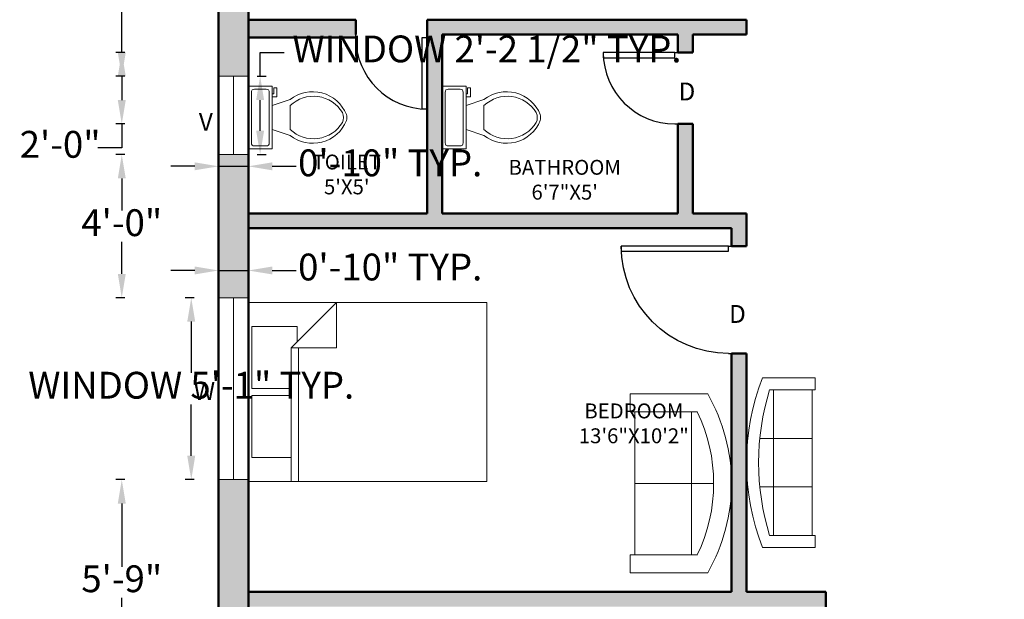
# Model space of a CAD drawing. Units: inches. Extents: x 2568 to 3190, y 746 to 1467.
# Tile 5 of 7: x 2568 to 2898, y 1073 to 1267. Entities that reach past the tile are written whole.
import ezdxf

# ---------------------------------------------------------------- set-up
doc = ezdxf.new("R2010")
doc.units = ezdxf.units.IN
for name, color, linetype, lineweight in [('A-ANNO-DIMS', 2, 'Continuous', 18), ('A-ANNO-TEXT', 7, 'Continuous', 18), ('A-AREA-IDEN', 7, 'Continuous', 25), ('A-DOOR', 3, 'Continuous', 25), ('A-FLOR-FIXT', 9, 'Continuous', 20), ('A-FURN', 8, 'Continuous', 18), ('A-GLAZ', 4, 'Continuous', 20), ('A-WALL', 7, 'Continuous', 50), ('A-WALL-PATT', 252, 'Continuous', 13)]:
    doc.layers.add(name, color=color, linetype=linetype, lineweight=lineweight)
doc.styles.get("Standard").update_dxf_attribs({"font": 'arial.ttf'})
doc.dimstyles.new('ISO-25', dxfattribs={"dimtxt": 9, "dimasz": 8, "dimexe": 2, "dimexo": 1, "dimtad": 0, "dimtih": 1, "dimtoh": 1, "dimdec": 1, "dimlunit": 3, "dimtxsty": 'Standard', "dimcen": 2.5, "dimclrd": 1, "dimclre": 3, "dimclrt": 6, "dimadec": 0, "dimazin": 0, "dimtfac": 1, "dimtdec": 1, "dimtmove": 0, "dimatfit": 3, "dimfxl": 1, "dimfxlon": 1, "dimarcsym": 0})

# ---------------------------------------------------------------- blocks, each defined once
blk = doc.blocks.new('*U2')
for p, q in [((-24, 0), (-24, -6)), ((0, 0), (0, -6))]:
    blk.add_line(p, q)
blk.add_lwpolyline([(0, 0), (0, 24), (-1.75, 24), (-1.75, 0)], close=True)
blk.add_arc((0, 0), 24, 90, 180)
blk = doc.blocks.new('*U5')
for p, q in [((-24, 0), (-24, 6)), ((0, 0), (0, 6))]:
    blk.add_line(p, q)
blk.add_lwpolyline([(0, 0), (0, -24), (-1.75, -24), (-1.75, 0)], close=True)
blk.add_arc((0, 0), 24, 180, 270)
blk = doc.blocks.new('*U7')
for p, q in [((0, 0), (0, -6)), ((36, 0), (36, -6))]:
    blk.add_line(p, q)
blk.add_lwpolyline([(0, 0), (0, 36), (1.75, 36), (1.75, 0)], close=True)
blk.add_arc((0, 0), 36, 0, 90)
blk = doc.blocks.new('Bed - Queen')
for p, q in [((0, -80.00003), (0, 0)), ((0, 0), (59.99999, 0)), ((59.99999, 0), (59.99999, -80.00003)), ((7.99999, -1.2), (28.79998, -1.2)), ((7.99999, -14.4), (7.99999, -1.2)), ((28.79998, -1.2), (28.79998, -14.4)), ((31.19999, -1.2), (51.99999, -1.2)), ((31.19999, -14.4), (31.19999, -1.2)), ((51.99999, -1.2), (51.99999, -16.4)), ((0, -14.4), (44.8, -14.4)), ((59.99999, -29.6), (44.8, -14.4)), ((44.8, -14.4), (44.8, -29.6)), ((51.99999, -16.4), (46.79936, -16.4)), ((44.8, -16.8), (0, -16.8)), ((44.8, -29.6), (59.99999, -29.6)), ((59.99999, -80.00003), (0, -80.00003))]:
    blk.add_line(p, q)
blk = doc.blocks.new('Sofa - Roundback 7 ft.')
for p, q in [((-12.00002, -32.4421), (-12.00003, -6.5971)), ((11.99997, -32.4421), (11.99998, -6.5971)), ((-36.000027, -34), (-36.000027, -11.4696)), ((-35.999844, -13.3819), (35.9998, -13.3819)), ((35.99998, -34), (35.99998, -11.4696)), ((-36.000027, -32.4421), (35.99998, -32.4421))]:
    blk.add_line(p, q)
for points in [[(-36.000027, -34), (-42.000027, -34), (-42.000027, -8)], [(41.99998, -8), (41.99998, -34), (35.99998, -34)]]:
    blk.add_lwpolyline(points)
for centre, radius, start, end in [((0, -114.25), 114.25, 68.43141, 111.5686), ((-0.00001, -127.1968), 121.1968, 72.72033, 107.2797)]:
    blk.add_arc(centre, radius, start, end)
blk = doc.blocks.new('Toilet - top')
for p, q in [((9.5, -6), (9.5, -2)), ((-10, -8.5), (-8, -8.5)), ((-10, -9.5), (-10, -8.5)), ((-7, -9.5), (-10, -9.5)), ((-8, -8.5), (-8, -8)), ((-7, -8), (-7, -9.5)), ((-4, -8), (-6, -14)), ((4, -8), (6, -14)), ((4, -14), (-4, -14))]:
    blk.add_line(p, q)
blk.add_lwpolyline([(10.5, -8), (10.5, 0), (-10.5, 0), (-10.5, -8)], close=True)
for points in [[(-9.5, -2), (-9.5, -6)], [(8.5, -1), (-8.5, -1)], [(-8.5, -7), (8.5, -7)]]:
    blk.add_lwpolyline(points)
for centre, radius, start, end in [((-8.62, -1.88), 0.884, 81.8699, 188.1301), ((8.62, -1.88), 0.884, 351.8699, 98.1301), ((-8.62, -6.12), 0.884, 171.8699, 278.1301), ((8.62, -6.12), 0.884, 261.8699, 8.1301), ((3.52, -21.58), 12.17, 141.4691, 247.9714), ((4.2, -21.82), 11.33, 136.3677, 238.9468), ((-3.52, -21.58), 12.17, 292.0284, 38.5307), ((-4.2, -21.82), 11.33, 301.053, 43.6321), ((0, -27.88), 4, 245.7318, 294.2682), ((0, -29), 4, 254.8605, 285.1395)]:
    blk.add_arc(centre, radius, start, end)
blk = doc.blocks.new('Sofa - Roundback Loveseat 5 ft.')
for p, q in [((0, -32.44198), (0, -5.99998)), ((-24, -33.99998), (-24, -11.46958)), ((24.00004, -33.99998), (24.00004, -11.46958)), ((-23.9998, -13.38178), (23.99986, -13.38178)), ((-24, -32.44198), (24.00004, -32.44198))]:
    blk.add_line(p, q)
for points in [[(-24, -33.99998), (-30, -33.99998), (-30, -7.99998)], [(30.00004, -7.99998), (30.00004, -33.99998), (24.00004, -33.99998)]]:
    blk.add_lwpolyline(points)
for centre, radius, start, end in [((0, -60.24998), 60.24998, 60.13715, 119.8628), ((0, -61.38438), 55.38444, 64.32083, 115.6792)]:
    blk.add_arc(centre, radius, start, end)
blk = doc.blocks.new('WIN-BATH-26.28')
for p, q in [((5, 26.28), (-5, 26.28)), ((0, 0), (0, 26.28)), ((5, 0), (-5, 0))]:
    blk.add_line(p, q)
blk = doc.blocks.new('WIN-BED-MIDDLE-61.03')
for p, q in [((5, 61.03), (-5, 61.03)), ((0, 61.03), (0, 0)), ((5, 0), (-5, 0))]:
    blk.add_line(p, q)
blk = doc.blocks.new('*D31')
at = {"layer": 'A-ANNO-DIMS', "color": 1, "lineweight": -2, "transparency": 16777216}
for p, q in [((2648.47, 1248.37), (2648.47, 1256.37)), ((2648.47, 1256.37), (2656.47, 1256.37)), ((2648.47, 1230.08), (2648.47, 1240.37))]:
    blk.add_line(p, q, dxfattribs=at)
at = {"layer": 'A-ANNO-DIMS', "color": 3, "lineweight": -2, "transparency": 16777216}
for p, q in [((2647.47, 1248.37), (2650.47, 1248.37)), ((2647.47, 1222.08), (2650.47, 1222.08))]:
    blk.add_line(p, q, dxfattribs=at)
at = {"layer": 'A-ANNO-DIMS', "color": 1, "transparency": 16777216}
for points in [[(2647.13, 1240.37), (2649.8, 1240.37), (2648.47, 1248.37)], [(2647.13, 1230.08), (2649.8, 1230.08), (2648.47, 1222.08)]]:
    blk.add_solid(points, dxfattribs=at)
at = {"layer": 'Defpoints', "color": 0, "transparency": 16777216}
for p in [(2644.52, 1248.37), (2648.47, 1248.37), (2644.52, 1222.08)]:
    blk.add_point(p, dxfattribs=at)
at = {"layer": 'A-ANNO-DIMS', "color": 6, "transparency": 16777216, "insert": (2724.52, 1256.37), "char_height": 9, "attachment_point": 5}
blk.add_mtext('WINDOW 2\'-2 1/2" TYP.', dxfattribs=at)
blk = doc.blocks.new('*D32')
at = {"layer": 'A-ANNO-DIMS', "color": 3, "lineweight": -2, "transparency": 16777216}
for p, q in [((2634.52, 1219.14), (2634.52, 1216.14)), ((2644.52, 1219.14), (2644.52, 1216.14))]:
    blk.add_line(p, q, dxfattribs=at)
at = {"layer": 'A-ANNO-DIMS', "color": 1, "lineweight": -2, "transparency": 16777216}
for p, q in [((2626.52, 1218.14), (2618.52, 1218.14)), ((2634.52, 1218.14), (2644.52, 1218.14)), ((2652.52, 1218.14), (2660.52, 1218.14))]:
    blk.add_line(p, q, dxfattribs=at)
at = {"layer": 'A-ANNO-DIMS', "color": 1, "transparency": 16777216}
for points in [[(2626.52, 1219.47), (2626.52, 1216.81), (2634.52, 1218.14)], [(2652.52, 1219.47), (2652.52, 1216.81), (2644.52, 1218.14)]]:
    blk.add_solid(points, dxfattribs=at)
at = {"layer": 'Defpoints', "color": 0, "transparency": 16777216}
for p in [(2634.52, 1222.08), (2644.52, 1222.08), (2644.52, 1218.14)]:
    blk.add_point(p, dxfattribs=at)
at = {"layer": 'A-ANNO-DIMS', "color": 6, "transparency": 16777216, "insert": (2692.07, 1218.14), "char_height": 9, "attachment_point": 5}
blk.add_mtext('0\'-10" TYP.', dxfattribs=at)
blk = doc.blocks.new('*D33')
at = {"layer": 'A-ANNO-DIMS', "color": 3, "lineweight": -2, "transparency": 16777216}
for p, q in [((2626.37, 1174.04), (2623.37, 1174.04)), ((2626.37, 1113), (2623.37, 1113))]:
    blk.add_line(p, q, dxfattribs=at)
at = {"layer": 'A-ANNO-DIMS', "color": 1, "lineweight": -2, "transparency": 16777216}
for p, q in [((2625.37, 1166.04), (2625.37, 1148.8)), ((2625.37, 1121), (2625.37, 1138.24))]:
    blk.add_line(p, q, dxfattribs=at)
at = {"layer": 'A-ANNO-DIMS', "color": 1, "transparency": 16777216}
for points in [[(2624.03, 1166.04), (2626.7, 1166.04), (2625.37, 1174.04)], [(2624.03, 1121), (2626.7, 1121), (2625.37, 1113)]]:
    blk.add_solid(points, dxfattribs=at)
at = {"layer": 'Defpoints', "color": 0, "transparency": 16777216}
for p in [(2625.37, 1174.04), (2634.52, 1174.04), (2634.52, 1113)]:
    blk.add_point(p, dxfattribs=at)
at = {"layer": 'A-ANNO-DIMS', "color": 6, "transparency": 16777216, "insert": (2625.37, 1143.52), "char_height": 9, "attachment_point": 5}
blk.add_mtext('WINDOW 5\'-1" TYP.', dxfattribs=at)
blk = doc.blocks.new('*D34')
at = {"layer": 'A-ANNO-DIMS', "color": 3, "lineweight": -2, "transparency": 16777216}
for p, q in [((2634.52, 1182.19), (2634.52, 1185.19)), ((2644.52, 1182.19), (2644.52, 1185.19))]:
    blk.add_line(p, q, dxfattribs=at)
at = {"layer": 'A-ANNO-DIMS', "color": 1, "lineweight": -2, "transparency": 16777216}
for p, q in [((2626.52, 1183.19), (2618.52, 1183.19)), ((2634.52, 1183.19), (2644.52, 1183.19)), ((2652.52, 1183.19), (2660.52, 1183.19))]:
    blk.add_line(p, q, dxfattribs=at)
at = {"layer": 'A-ANNO-DIMS', "color": 1, "transparency": 16777216}
for points in [[(2626.52, 1184.53), (2626.52, 1181.86), (2634.52, 1183.19)], [(2652.52, 1184.53), (2652.52, 1181.86), (2644.52, 1183.19)]]:
    blk.add_solid(points, dxfattribs=at)
at = {"layer": 'Defpoints', "color": 0, "transparency": 16777216}
for p in [(2644.52, 1183.19), (2634.52, 1174.04), (2644.52, 1174.04)]:
    blk.add_point(p, dxfattribs=at)
at = {"layer": 'A-ANNO-DIMS', "color": 6, "transparency": 16777216, "insert": (2692.07, 1183.19), "char_height": 9, "attachment_point": 5}
blk.add_mtext('0\'-10" TYP.', dxfattribs=at)
blk = doc.blocks.new('*D39')
at = {"layer": 'A-ANNO-DIMS', "color": 3, "lineweight": -2, "transparency": 16777216}
for p, q in [((2644.52, 760.85), (2644.52, 757.85)), ((2709.74, 760.85), (2709.74, 757.85))]:
    blk.add_line(p, q, dxfattribs=at)
at = {"layer": 'A-ANNO-DIMS', "color": 1, "lineweight": -2, "transparency": 16777216}
for p, q in [((2652.52, 759.85), (2664.54, 759.85)), ((2701.74, 759.85), (2689.72, 759.85))]:
    blk.add_line(p, q, dxfattribs=at)
at = {"layer": 'A-ANNO-DIMS', "color": 1, "transparency": 16777216}
for points in [[(2652.52, 761.18), (2652.52, 758.51), (2644.52, 759.85)], [(2701.74, 761.18), (2701.74, 758.51), (2709.74, 759.85)]]:
    blk.add_solid(points, dxfattribs=at)
at = {"layer": 'Defpoints', "color": 0, "transparency": 16777216}
for p in [(2644.52, 1411.35), (2709.74, 1411.35), (2709.74, 759.85)]:
    blk.add_point(p, dxfattribs=at)
at = {"layer": 'A-ANNO-DIMS', "color": 6, "transparency": 16777216, "insert": (2677.13, 759.85), "char_height": 9, "attachment_point": 5}
blk.add_mtext('5\'-5"', dxfattribs=at)
blk = doc.blocks.new('*D40')
at = {"layer": 'A-ANNO-DIMS', "color": 3, "lineweight": -2, "transparency": 16777216}
for p, q in [((2709.74, 760.85), (2709.74, 757.85)), ((2763.78, 760.85), (2763.78, 757.85))]:
    blk.add_line(p, q, dxfattribs=at)
at = {"layer": 'A-ANNO-DIMS', "color": 1, "lineweight": -2, "transparency": 16777216}
for p, q in [((2717.74, 759.85), (2723.99, 759.85)), ((2755.78, 759.85), (2749.52, 759.85))]:
    blk.add_line(p, q, dxfattribs=at)
at = {"layer": 'A-ANNO-DIMS', "color": 1, "transparency": 16777216}
for points in [[(2717.74, 761.18), (2717.74, 758.51), (2709.74, 759.85)], [(2755.78, 761.18), (2755.78, 758.51), (2763.78, 759.85)]]:
    blk.add_solid(points, dxfattribs=at)
at = {"layer": 'Defpoints', "color": 0, "transparency": 16777216}
for p in [(2709.74, 1411.35), (2763.78, 1411.35), (2763.78, 759.85)]:
    blk.add_point(p, dxfattribs=at)
at = {"layer": 'A-ANNO-DIMS', "color": 6, "transparency": 16777216, "insert": (2736.76, 759.85), "char_height": 9, "attachment_point": 5}
blk.add_mtext('4\'-6"', dxfattribs=at)
blk = doc.blocks.new('*D41')
at = {"layer": 'A-ANNO-DIMS', "color": 1, "lineweight": -2, "transparency": 16777216}
for p, q in [((2803.52, 759.85), (2795.52, 759.85)), ((2811.52, 759.85), (2815.43, 759.85)), ((2844.66, 759.85), (2840.76, 759.85)), ((2852.66, 759.85), (2860.66, 759.85))]:
    blk.add_line(p, q, dxfattribs=at)
at = {"layer": 'A-ANNO-DIMS', "color": 3, "lineweight": -2, "transparency": 16777216}
for p, q in [((2811.52, 760.85), (2811.52, 757.85)), ((2844.66, 760.85), (2844.66, 757.85))]:
    blk.add_line(p, q, dxfattribs=at)
at = {"layer": 'A-ANNO-DIMS', "color": 1, "transparency": 16777216}
for points in [[(2803.52, 761.18), (2803.52, 758.51), (2811.52, 759.85)], [(2852.66, 761.18), (2852.66, 758.51), (2844.66, 759.85)]]:
    blk.add_solid(points, dxfattribs=at)
at = {"layer": 'Defpoints', "color": 0, "transparency": 16777216}
for p in [(2811.52, 1411.35), (2844.66, 1411.35), (2844.66, 759.85)]:
    blk.add_point(p, dxfattribs=at)
at = {"layer": 'A-ANNO-DIMS', "color": 6, "transparency": 16777216, "insert": (2828.09, 759.85), "char_height": 9, "attachment_point": 5}
blk.add_mtext('2\'-9"', dxfattribs=at)
blk = doc.blocks.new('*D42')
at = {"layer": 'A-ANNO-DIMS', "color": 3, "lineweight": -2, "transparency": 16777216}
for p, q in [((2844.66, 760.85), (2844.66, 757.85)), ((2897.43, 760.85), (2897.43, 757.85))]:
    blk.add_line(p, q, dxfattribs=at)
at = {"layer": 'A-ANNO-DIMS', "color": 1, "lineweight": -2, "transparency": 16777216}
for p, q in [((2852.66, 759.85), (2858.28, 759.85)), ((2889.43, 759.85), (2883.81, 759.85))]:
    blk.add_line(p, q, dxfattribs=at)
at = {"layer": 'A-ANNO-DIMS', "color": 1, "transparency": 16777216}
for points in [[(2852.66, 761.18), (2852.66, 758.51), (2844.66, 759.85)], [(2889.43, 761.18), (2889.43, 758.51), (2897.43, 759.85)]]:
    blk.add_solid(points, dxfattribs=at)
at = {"layer": 'Defpoints', "color": 0, "transparency": 16777216}
for p in [(2844.66, 1411.35), (2897.43, 1411.35), (2897.43, 759.85)]:
    blk.add_point(p, dxfattribs=at)
at = {"layer": 'A-ANNO-DIMS', "color": 6, "transparency": 16777216, "insert": (2871.04, 759.85), "char_height": 9, "attachment_point": 5}
blk.add_mtext('4\'-5"', dxfattribs=at)
blk = doc.blocks.new('*D47')
at = {"layer": 'A-ANNO-DIMS', "color": 3, "lineweight": -2, "transparency": 16777216}
for p, q in [((2754.37, 1452.8), (2754.37, 1455.8)), ((2846.86, 1452.8), (2846.86, 1455.8))]:
    blk.add_line(p, q, dxfattribs=at)
at = {"layer": 'A-ANNO-DIMS', "color": 1, "lineweight": -2, "transparency": 16777216}
for p, q in [((2762.37, 1453.8), (2777.58, 1453.8)), ((2838.86, 1453.8), (2823.65, 1453.8))]:
    blk.add_line(p, q, dxfattribs=at)
at = {"layer": 'A-ANNO-DIMS', "color": 1, "transparency": 16777216}
for points in [[(2762.37, 1455.13), (2762.37, 1452.47), (2754.37, 1453.8)], [(2838.86, 1455.13), (2838.86, 1452.47), (2846.86, 1453.8)]]:
    blk.add_solid(points, dxfattribs=at)
at = {"layer": 'Defpoints', "color": 0, "transparency": 16777216}
for p in [(2846.86, 1453.8), (2754.37, 831.35), (2846.86, 831.35)]:
    blk.add_point(p, dxfattribs=at)
at = {"layer": 'A-ANNO-DIMS', "color": 6, "transparency": 16777216, "insert": (2800.61, 1453.8), "char_height": 9, "attachment_point": 5}
blk.add_mtext('7\'-8 1/2"', dxfattribs=at)
blk = doc.blocks.new('*D50')
at = {"layer": 'A-ANNO-DIMS', "color": 1, "lineweight": -2, "transparency": 16777216}
for p, q in [((2838.86, 1453.8), (2830.86, 1453.8)), ((2846.86, 1453.8), (2851.29, 1453.8)), ((2902.21, 1453.8), (2897.79, 1453.8)), ((2910.21, 1453.8), (2918.21, 1453.8))]:
    blk.add_line(p, q, dxfattribs=at)
at = {"layer": 'A-ANNO-DIMS', "color": 3, "lineweight": -2, "transparency": 16777216}
for p, q in [((2846.86, 1452.8), (2846.86, 1455.8)), ((2902.21, 1452.8), (2902.21, 1455.8))]:
    blk.add_line(p, q, dxfattribs=at)
at = {"layer": 'A-ANNO-DIMS', "color": 1, "transparency": 16777216}
for points in [[(2838.86, 1455.13), (2838.86, 1452.47), (2846.86, 1453.8)], [(2910.21, 1455.13), (2910.21, 1452.47), (2902.21, 1453.8)]]:
    blk.add_solid(points, dxfattribs=at)
at = {"layer": 'Defpoints', "color": 0, "transparency": 16777216}
for p in [(2902.21, 1453.8), (2846.86, 831.35), (2902.21, 831.35)]:
    blk.add_point(p, dxfattribs=at)
at = {"layer": 'A-ANNO-DIMS', "color": 6, "transparency": 16777216, "insert": (2874.54, 1453.8), "char_height": 9, "attachment_point": 5}
blk.add_mtext('4\'-7 1/2"', dxfattribs=at)
blk = doc.blocks.new('*D54')
at = {"layer": 'A-ANNO-DIMS', "color": 3, "lineweight": -2, "transparency": 16777216}
for p, q in [((2850.52, 760.85), (2850.52, 757.85)), ((2898.52, 760.85), (2898.52, 757.85))]:
    blk.add_line(p, q, dxfattribs=at)
at = {"layer": 'A-ANNO-DIMS', "color": 1, "lineweight": -2, "transparency": 16777216}
for p, q in [((2858.52, 759.85), (2861.75, 759.85)), ((2890.52, 759.85), (2887.29, 759.85))]:
    blk.add_line(p, q, dxfattribs=at)
at = {"layer": 'A-ANNO-DIMS', "color": 1, "transparency": 16777216}
for points in [[(2858.52, 761.18), (2858.52, 758.51), (2850.52, 759.85)], [(2890.52, 761.18), (2890.52, 758.51), (2898.52, 759.85)]]:
    blk.add_solid(points, dxfattribs=at)
at = {"layer": 'Defpoints', "color": 0, "transparency": 16777216}
for p in [(2850.52, 1310.35), (2898.52, 1310.35), (2898.52, 759.85)]:
    blk.add_point(p, dxfattribs=at)
at = {"layer": 'A-ANNO-DIMS', "color": 6, "transparency": 16777216, "insert": (2874.52, 759.85), "char_height": 9, "attachment_point": 5}
blk.add_mtext('4\'-0"', dxfattribs=at)
blk = doc.blocks.new('*D64')
at = {"layer": 'A-ANNO-DIMS', "color": 1, "lineweight": -2, "transparency": 16777216}
for p, q in [((2636.52, 759.85), (2628.52, 759.85)), ((2644.52, 759.85), (2649.94, 759.85)), ((2680.52, 759.85), (2675.11, 759.85)), ((2688.52, 759.85), (2696.52, 759.85))]:
    blk.add_line(p, q, dxfattribs=at)
at = {"layer": 'A-ANNO-DIMS', "color": 3, "lineweight": -2, "transparency": 16777216}
for p, q in [((2644.52, 760.85), (2644.52, 757.85)), ((2680.52, 760.85), (2680.52, 757.85))]:
    blk.add_line(p, q, dxfattribs=at)
at = {"layer": 'A-ANNO-DIMS', "color": 1, "transparency": 16777216}
for points in [[(2636.52, 761.18), (2636.52, 758.51), (2644.52, 759.85)], [(2688.52, 761.18), (2688.52, 758.51), (2680.52, 759.85)]]:
    blk.add_solid(points, dxfattribs=at)
at = {"layer": 'Defpoints', "color": 0, "transparency": 16777216}
for p in [(2644.52, 1261.35), (2680.52, 1262.35), (2680.52, 759.85)]:
    blk.add_point(p, dxfattribs=at)
at = {"layer": 'A-ANNO-DIMS', "color": 6, "transparency": 16777216, "insert": (2662.52, 759.85), "char_height": 9, "attachment_point": 5}
blk.add_mtext('3\'-0"', dxfattribs=at)
blk = doc.blocks.new('*D65')
at = {"layer": 'A-ANNO-DIMS', "color": 3, "lineweight": -2, "transparency": 16777216}
for p, q in [((2680.52, 760.85), (2680.52, 757.85)), ((2704.52, 760.85), (2704.52, 757.85))]:
    blk.add_line(p, q, dxfattribs=at)
at = {"layer": 'A-ANNO-DIMS', "color": 1, "lineweight": -2, "transparency": 16777216}
for p, q in [((2688.52, 759.85), (2696.52, 759.85)), ((2704.52, 759.85), (2712.52, 759.85))]:
    blk.add_line(p, q, dxfattribs=at)
at = {"layer": 'A-ANNO-DIMS', "color": 1, "transparency": 16777216}
for points in [[(2688.52, 761.18), (2688.52, 758.51), (2680.52, 759.85)], [(2696.52, 761.18), (2696.52, 758.51), (2704.52, 759.85)]]:
    blk.add_solid(points, dxfattribs=at)
at = {"layer": 'Defpoints', "color": 0, "transparency": 16777216}
for p in [(2680.52, 1262.35), (2704.52, 1261.35), (2704.52, 759.85)]:
    blk.add_point(p, dxfattribs=at)
at = {"layer": 'A-ANNO-DIMS', "color": 6, "transparency": 16777216, "insert": (2725.19, 759.85), "char_height": 9, "attachment_point": 5}
blk.add_mtext('2\'-0"', dxfattribs=at)
blk = doc.blocks.new('*D69')
at = {"layer": 'A-ANNO-DIMS', "color": 3, "lineweight": -2, "transparency": 16777216}
for p, q in [((2603.07, 1113), (2600.07, 1113)), ((2603.07, 1044.16), (2600.07, 1044.16))]:
    blk.add_line(p, q, dxfattribs=at)
at = {"layer": 'A-ANNO-DIMS', "color": 1, "lineweight": -2, "transparency": 16777216}
for p, q in [((2602.07, 1105), (2602.07, 1083.8)), ((2602.07, 1052.16), (2602.07, 1073.36))]:
    blk.add_line(p, q, dxfattribs=at)
at = {"layer": 'A-ANNO-DIMS', "color": 1, "transparency": 16777216}
for points in [[(2600.74, 1105), (2603.41, 1105), (2602.07, 1113)], [(2600.74, 1052.16), (2603.41, 1052.16), (2602.07, 1044.16)]]:
    blk.add_solid(points, dxfattribs=at)
at = {"layer": 'Defpoints', "color": 0, "transparency": 16777216}
for p in [(2602.07, 1113), (2634.52, 1113), (2634.52, 1044.16)]:
    blk.add_point(p, dxfattribs=at)
at = {"layer": 'A-ANNO-DIMS', "color": 6, "transparency": 16777216, "insert": (2602.07, 1078.58), "char_height": 9, "attachment_point": 5}
blk.add_mtext('5\'-9"', dxfattribs=at)
blk = doc.blocks.new('*D70')
at = {"layer": 'A-ANNO-DIMS', "color": 3, "lineweight": -2, "transparency": 16777216}
for p, q in [((2603.07, 1222.08), (2600.07, 1222.08)), ((2603.07, 1174.04), (2600.07, 1174.04))]:
    blk.add_line(p, q, dxfattribs=at)
at = {"layer": 'A-ANNO-DIMS', "color": 1, "lineweight": -2, "transparency": 16777216}
for p, q in [((2602.07, 1214.08), (2602.07, 1203.28)), ((2602.07, 1182.04), (2602.07, 1192.84))]:
    blk.add_line(p, q, dxfattribs=at)
at = {"layer": 'A-ANNO-DIMS', "color": 1, "transparency": 16777216}
for points in [[(2600.74, 1214.08), (2603.41, 1214.08), (2602.07, 1222.08)], [(2600.74, 1182.04), (2603.41, 1182.04), (2602.07, 1174.04)]]:
    blk.add_solid(points, dxfattribs=at)
at = {"layer": 'Defpoints', "color": 0, "transparency": 16777216}
for p in [(2602.07, 1222.08), (2634.52, 1222.08), (2634.52, 1174.04)]:
    blk.add_point(p, dxfattribs=at)
at = {"layer": 'A-ANNO-DIMS', "color": 6, "transparency": 16777216, "insert": (2602.07, 1198.06), "char_height": 9, "attachment_point": 5}
blk.add_mtext('4\'-0"', dxfattribs=at)
blk = doc.blocks.new('*D71')
at = {"layer": 'A-ANNO-DIMS', "color": 3, "lineweight": -2, "transparency": 16777216}
for p, q in [((2603.07, 1316.62), (2600.07, 1316.62)), ((2603.07, 1248.37), (2600.07, 1248.37))]:
    blk.add_line(p, q, dxfattribs=at)
at = {"layer": 'A-ANNO-DIMS', "color": 1, "lineweight": -2, "transparency": 16777216}
for p, q in [((2602.07, 1308.62), (2602.07, 1287.71)), ((2602.07, 1256.37), (2602.07, 1277.27))]:
    blk.add_line(p, q, dxfattribs=at)
at = {"layer": 'A-ANNO-DIMS', "color": 1, "transparency": 16777216}
for points in [[(2600.74, 1308.62), (2603.41, 1308.62), (2602.07, 1316.62)], [(2600.74, 1256.37), (2603.41, 1256.37), (2602.07, 1248.37)]]:
    blk.add_solid(points, dxfattribs=at)
at = {"layer": 'Defpoints', "color": 0, "transparency": 16777216}
for p in [(2602.07, 1316.62), (2634.52, 1316.62), (2634.52, 1248.37)]:
    blk.add_point(p, dxfattribs=at)
at = {"layer": 'A-ANNO-DIMS', "color": 6, "transparency": 16777216, "insert": (2602.07, 1282.49), "char_height": 9, "attachment_point": 5}
blk.add_mtext('5\'-8"', dxfattribs=at)
blk = doc.blocks.new('*D78')
at = {"layer": 'A-ANNO-DIMS', "color": 3, "lineweight": -2, "transparency": 16777216}
for p, q in [((2603.07, 1256.35), (2600.07, 1256.35)), ((2603.07, 1232.35), (2600.07, 1232.35))]:
    blk.add_line(p, q, dxfattribs=at)
at = {"layer": 'A-ANNO-DIMS', "color": 1, "lineweight": -2, "transparency": 16777216}
for p, q in [((2602.07, 1248.35), (2602.07, 1240.35)), ((2602.07, 1232.35), (2602.07, 1224.35)), ((2602.07, 1224.35), (2594.07, 1224.35))]:
    blk.add_line(p, q, dxfattribs=at)
at = {"layer": 'A-ANNO-DIMS', "color": 1, "transparency": 16777216}
for points in [[(2600.74, 1248.35), (2603.41, 1248.35), (2602.07, 1256.35)], [(2600.74, 1240.35), (2603.41, 1240.35), (2602.07, 1232.35)]]:
    blk.add_solid(points, dxfattribs=at)
at = {"layer": 'Defpoints', "color": 0, "transparency": 16777216}
for p in [(2955.52, 1256.35), (2602.07, 1232.35), (2955.52, 1232.35)]:
    blk.add_point(p, dxfattribs=at)
at = {"layer": 'A-ANNO-DIMS', "color": 6, "transparency": 16777216, "insert": (2581.41, 1224.35), "char_height": 9, "attachment_point": 5}
blk.add_mtext('2\'-0"', dxfattribs=at)
blk = doc.blocks.new('*D80')
at = {"layer": 'A-ANNO-DIMS', "color": 3, "lineweight": -2, "transparency": 16777216}
for p, q in [((2838.1, 1452.8), (2838.1, 1455.8)), ((2910.92, 1452.8), (2910.92, 1455.8))]:
    blk.add_line(p, q, dxfattribs=at)
at = {"layer": 'A-ANNO-DIMS', "color": 1, "lineweight": -2, "transparency": 16777216}
for p, q in [((2846.1, 1453.8), (2861.9, 1453.8)), ((2902.92, 1453.8), (2887.12, 1453.8))]:
    blk.add_line(p, q, dxfattribs=at)
at = {"layer": 'A-ANNO-DIMS', "color": 1, "transparency": 16777216}
for points in [[(2846.1, 1455.13), (2846.1, 1452.47), (2838.1, 1453.8)], [(2902.92, 1455.13), (2902.92, 1452.47), (2910.92, 1453.8)]]:
    blk.add_solid(points, dxfattribs=at)
at = {"layer": 'Defpoints', "color": 0, "transparency": 16777216}
for p in [(2910.92, 1453.8), (2838.1, 1075.35), (2910.92, 1075.35)]:
    blk.add_point(p, dxfattribs=at)
at = {"layer": 'A-ANNO-DIMS', "color": 6, "transparency": 16777216, "insert": (2874.51, 1453.8), "char_height": 9, "attachment_point": 5}
blk.add_mtext('6\'-1"', dxfattribs=at)
blk = doc.blocks.new('*D81')
at = {"layer": 'A-ANNO-DIMS', "color": 3, "lineweight": -2, "transparency": 16777216}
for p, q in [((2811.52, 1452.8), (2811.52, 1455.8)), ((2838.1, 1452.8), (2838.1, 1455.8))]:
    blk.add_line(p, q, dxfattribs=at)
at = {"layer": 'A-ANNO-DIMS', "color": 1, "lineweight": -2, "transparency": 16777216}
for p, q in [((2819.52, 1453.8), (2830.1, 1453.8)), ((2838.1, 1453.8), (2846.1, 1453.8))]:
    blk.add_line(p, q, dxfattribs=at)
at = {"layer": 'A-ANNO-DIMS', "color": 1, "transparency": 16777216}
for points in [[(2819.52, 1455.13), (2819.52, 1452.47), (2811.52, 1453.8)], [(2830.1, 1455.13), (2830.1, 1452.47), (2838.1, 1453.8)]]:
    blk.add_solid(points, dxfattribs=at)
at = {"layer": 'Defpoints', "color": 0, "transparency": 16777216}
for p in [(2838.1, 1453.8), (2811.52, 1075.35), (2838.1, 1075.35)]:
    blk.add_point(p, dxfattribs=at)
at = {"layer": 'A-ANNO-DIMS', "color": 6, "transparency": 16777216, "insert": (2869.24, 1453.8), "char_height": 9, "attachment_point": 5}
blk.add_mtext('2\'-2 1/2"', dxfattribs=at)

msp = doc.modelspace()

# ---------------------------------------------------------------- hatches: boundary and pattern name
at = {"layer": 'A-WALL-PATT'}
h = msp.add_hatch(color=256, dxfattribs=at)
h.dxf.hatch_style = 1
h.paths.add_polyline_path([(2709.74, 1411.35), (2709.74, 1421.35), (2634.52, 1421.35), (2634.52, 1371.08), (2644.52, 1371.08), (2644.52, 1411.35)])
h.paths.add_polyline_path([(2844.66, 1411.35), (2844.66, 1421.35), (2763.78, 1421.35), (2763.78, 1411.35)])
h.paths.add_polyline_path([(2996.2, 1411.35), (2996.2, 1421.35), (2897.43, 1421.35), (2897.43, 1411.35)])
h.paths.add_polyline_path([(3104.52, 1411.35), (3104.52, 1371.08), (3114.52, 1371.08), (3114.52, 1421.35), (3052.64, 1421.35), (3052.64, 1411.35)])
h.paths.add_polyline_path([(3114.52, 1316.62), (3104.52, 1316.62), (3104.52, 1248.37), (3114.52, 1248.37)])
h.paths.add_polyline_path([(3104.52, 1174.04), (3114.52, 1174.04), (3114.52, 1222.08), (3104.52, 1222.08)])
h.paths.add_polyline_path([(3104.52, 1020.11), (3114.52, 1020.11), (3114.52, 1113), (3104.52, 1113)])
h.paths.add_polyline_path([(3104.52, 920.42), (3114.52, 920.42), (3114.52, 992.96), (3104.52, 992.96)])
h.paths.add_polyline_path([(3114.52, 821.35), (3114.52, 865.93), (3104.52, 865.93), (3104.52, 831.35), (3055.78, 831.35), (3055.78, 821.35)])
h.paths.add_polyline_path([(2902.21, 831.35), (2902.21, 821.35), (2986.63, 821.35), (2986.63, 831.35)])
h.paths.add_polyline_path([(2634.52, 821.35), (2676.76, 821.35), (2676.76, 831.35), (2644.52, 831.35), (2644.52, 865.93), (2634.52, 865.93)])
h.paths.add_polyline_path([(2754.37, 821.35), (2846.86, 821.35), (2846.86, 831.35), (2754.37, 831.35)])
h.paths.add_polyline_path([(2644.52, 920.42), (2644.52, 1002.57), (2634.52, 1002.57), (2634.52, 920.42)])
h.paths.add_polyline_path([(2644.52, 1044.16), (2644.52, 1113), (2634.52, 1113), (2634.52, 1044.16)])
h.paths.add_polyline_path([(2644.52, 1248.37), (2644.52, 1316.62), (2634.52, 1316.62), (2634.52, 1248.37)])
h.paths.add_polyline_path([(2634.52, 1222.08), (2634.52, 1174.04), (2644.52, 1174.04), (2644.52, 1222.08)])
h = msp.add_hatch(color=256, dxfattribs=at)
h.dxf.hatch_style = 1
h.paths.add_polyline_path([(2811.52, 1411.35), (2806.52, 1411.35), (2806.52, 1303.35), (2811.52, 1303.35), (2811.52, 1310.35), (2850.52, 1310.35), (2850.52, 1315.35), (2811.52, 1315.35)])
h.paths.add_polyline_path([(2942.52, 1411.35), (2937.52, 1411.35), (2937.52, 1315.35), (2898.52, 1315.35), (2898.52, 1310.35), (2937.52, 1310.35), (2937.52, 1303.35), (2942.52, 1303.35)])
h.paths.add_polyline_path([(2811.52, 1267.35), (2704.52, 1267.35), (2704.52, 1261.35), (2704.52, 1237.35), (2704.52, 1202.35), (2644.52, 1202.35), (2644.52, 1197.35), (2806.52, 1197.35), (2806.52, 1191.38), (2811.52, 1191.38), (2811.52, 1202.35), (2793.52, 1202.35), (2793.52, 1232.35), (2788.52, 1232.35), (2788.52, 1202.35), (2709.52, 1202.35), (2709.52, 1262.35), (2788.52, 1262.35), (2788.52, 1256.35), (2793.52, 1256.35), (2793.52, 1262.35), (2811.52, 1262.35)])
h.paths.add_polyline_path([(2680.52, 1267.35), (2644.52, 1267.35), (2644.52, 1261.35), (2680.52, 1261.35)])
h.paths.add_polyline_path([(3044.52, 1267.35), (2937.52, 1267.35), (2937.52, 1262.35), (2955.52, 1262.35), (2955.52, 1256.35), (2960.52, 1256.35), (2960.52, 1262.35), (3039.52, 1262.35), (3039.52, 1202.35), (2960.52, 1202.35), (2960.52, 1232.35), (2955.52, 1232.35), (2955.52, 1202.35), (2937.52, 1202.35), (2937.52, 1191.38), (2942.52, 1191.38), (2942.52, 1197.35), (3104.52, 1197.35), (3104.52, 1202.35), (3044.52, 1202.35)])
h.paths.add_polyline_path([(3104.52, 1267.35), (3072.52, 1267.35), (3072.52, 1262.35), (3104.52, 1262.35)])
h.paths.add_polyline_path([(2838.1, 1075.35), (2811.52, 1075.35), (2811.52, 1155.35), (2806.52, 1155.35), (2806.52, 1075.35), (2644.52, 1075.35), (2644.52, 1070.35), (2806.52, 1070.35), (2811.52, 1070.35), (2838.1, 1070.35)])
h.paths.add_polyline_path([(3104.52, 1075.35), (2942.52, 1075.35), (2942.52, 1155.38), (2937.52, 1155.38), (2937.52, 1075.35), (2910.92, 1075.35), (2910.92, 1070.35), (2937.52, 1070.35), (3104.52, 1070.35)])
h.paths.add_polyline_path([(2811.52, 1038.35), (2806.52, 1038.35), (2806.52, 980.35), (2644.52, 980.35), (2644.52, 975.35), (2806.52, 975.35), (2806.52, 969.37), (2811.52, 969.37), (2811.52, 975.35)])
h.paths.add_polyline_path([(3104.52, 980.35), (2937.52, 980.35), (2937.52, 969.35), (2942.52, 969.35), (2942.52, 975.35), (3104.52, 975.35)])
h.paths.add_polyline_path([(3104.52, 1034.35), (3039.52, 1034.35), (3039.52, 1004.35), (3044.52, 1004.35), (3044.52, 1029.35), (3104.52, 1029.35)])
h.paths.add_polyline_path([(2942.52, 933.35), (2937.52, 933.35), (2937.52, 831.35), (2942.52, 831.35)])
h.paths.add_polyline_path([(2811.52, 933.37), (2806.52, 933.37), (2806.52, 831.35), (2811.52, 831.35)])

# ---------------------------------------------------------------- linework, layer by layer
at = {"layer": 'A-WALL'}
for p, q in [((2634.52, 1421.35), (2634.52, 821.35)), ((2644.52, 1411.35), (2644.52, 831.35)), ((2680.52, 1267.35), (2644.52, 1267.35)), ((2680.52, 1267.35), (2680.52, 1262.35)), ((2704.52, 1267.35), (2704.52, 1202.35)), ((2704.52, 1267.35), (2811.52, 1267.35)), ((2811.52, 1262.35), (2811.52, 1267.35)), ((2680.52, 1261.35), (2644.52, 1261.35)), ((2709.52, 1262.35), (2709.52, 1202.35)), ((2709.52, 1262.35), (2788.52, 1262.35)), ((2788.52, 1256.35), (2788.52, 1262.35)), ((2793.52, 1262.35), (2793.52, 1256.35)), ((2793.52, 1262.35), (2811.52, 1262.35)), ((2793.52, 1256.35), (2788.52, 1256.35)), ((2788.52, 1232.35), (2788.52, 1202.35)), ((2788.52, 1232.35), (2793.52, 1232.35)), ((2793.52, 1232.35), (2793.52, 1202.35)), ((2704.52, 1202.35), (2644.52, 1202.35)), ((2788.52, 1202.35), (2709.52, 1202.35)), ((2811.52, 1202.35), (2793.52, 1202.35)), ((2811.52, 1202.35), (2811.52, 1191.35)), ((2806.52, 1197.35), (2644.52, 1197.35)), ((2806.52, 1197.35), (2806.52, 1191.35)), ((2806.52, 1191.35), (2811.52, 1191.35)), ((2806.52, 1155.35), (2811.52, 1155.35)), ((2806.52, 1155.35), (2806.52, 1075.35)), ((2811.52, 1155.35), (2811.52, 1075.35)), ((2806.52, 1075.35), (2644.52, 1075.35)), ((2838.1, 1075.35), (2811.52, 1075.35)), ((2838.1, 1075.35), (2838.1, 1070.35))]:
    msp.add_line(p, q, dxfattribs=at)

# ---------------------------------------------------------------- block references
at = {"layer": 'A-DOOR'}
msp.add_blockref('*U5', (2704.52, 1261.35), dxfattribs=at)
at = {"layer": 'A-DOOR', "rotation": 90}
msp.add_blockref('*U2', (2787.52, 1256.35), dxfattribs=at)
at = {"layer": 'A-DOOR', "xscale": -1, "rotation": 90}
msp.add_blockref('*U7', (2805.52, 1191.38), dxfattribs=at)
at = {"layer": 'A-FLOR-FIXT', "xscale": -1, "rotation": 90}
for p in [(2644.52, 1234.51), (2709.52, 1234.51)]:
    msp.add_blockref('Toilet - top', p, dxfattribs=at)
at = {"layer": 'A-FURN'}
for name, p, rotation in [('Bed - Queen', (2644.52, 1112.43), 90), ('Sofa - Roundback Loveseat 5 ft.', (2806.52, 1111.75), 270)]:
    msp.add_blockref(name, p, dxfattribs=dict(at, rotation=rotation))
at = {"layer": 'A-FURN', "xscale": 0.6782133153273913, "yscale": 0.6782133153273913, "zscale": 0.6782133153273913, "rotation": 90}
msp.add_blockref('Sofa - Roundback 7 ft.', (2811.52, 1118.73), dxfattribs=at)
at = {"layer": 'A-GLAZ'}
for name, p in [('WIN-BATH-26.28', (2639.52, 1222.08)), ('WIN-BED-MIDDLE-61.03', (2639.52, 1113))]:
    msp.add_blockref(name, p, dxfattribs=at)

# ---------------------------------------------------------------- texts
at = {"layer": 'A-ANNO-TEXT', "char_height": 6, "attachment_point": 1}
for s, insert in [('D', (2788.74, 1246.25)), ('V', (2627.91, 1236.06)), ('D', (2805.68, 1171.6)), ('W', (2626.17, 1145.73))]:
    msp.add_mtext_dynamic_manual_height_columns(s, width=7.7602, gutter_width=12.5, heights=[0], dxfattribs=dict(at, insert=insert))
at = {"layer": 'A-AREA-IDEN', "char_height": 5, "attachment_point": 1}
for s, insert in [("\\pxqc;TOILET\\P5'X5'", (2642.58, 1222.08)), ('\\pxqc;BATHROOM\\P6\'7"X5\'', (2715.65, 1220.31)), ('\\pxqc;BEDROOM\\P13\'6"X10\'2"', (2738.83, 1138.56))]:
    msp.add_mtext_dynamic_manual_height_columns(s, width=69.8646, gutter_width=12.5, heights=[0], dxfattribs=dict(at, insert=insert))

# ---------------------------------------------------------------- dimensions: what is measured, and where the dimension line sits
at = {"layer": 'A-ANNO-DIMS'}
for base, p1, p2, picture, middle in [((2846.86, 1453.8), (2754.37, 831.35), (2846.86, 831.35), '*D47', (2800.61, 1453.8)), ((2838.1, 1453.8), (2811.52, 1075.35), (2838.1, 1075.35), '*D81', (2869.24, 1453.8)), ((2902.2147, 1453.7989), (2846.8636, 831.3489), (2902.2147, 831.3489), '*D50', (2874.5391, 1453.7989)), ((2910.92, 1453.8), (2838.1, 1075.35), (2910.92, 1075.35), '*D80', (2874.51, 1453.8)), ((2709.74, 759.85), (2644.52, 1411.35), (2709.74, 1411.35), '*D39', (2677.13, 759.85)), ((2763.78, 759.85), (2709.74, 1411.35), (2763.78, 1411.35), '*D40', (2736.76, 759.85)), ((2844.66, 759.85), (2811.52, 1411.35), (2844.66, 1411.35), '*D41', (2828.09, 759.85)), ((2897.43, 759.85), (2844.66, 1411.35), (2897.43, 1411.35), '*D42', (2871.04, 759.85)), ((2898.52, 759.85), (2850.52, 1310.35), (2898.52, 1310.35), '*D54', (2874.52, 759.85)), ((2680.52, 759.85), (2644.52, 1261.35), (2680.52, 1262.35), '*D64', (2662.52, 759.85)), ((2704.52, 759.85), (2680.52, 1262.35), (2704.52, 1261.35), '*D65', (2725.19, 759.85))]:
    dim = msp.add_linear_dim(base=base, p1=p1, p2=p2, dimstyle='ISO-25', override={"dimdec": 1, "dimlfac": 1, "dimrnd": 0, "dimzin": 1, "dimdsep": 46, "dimlunit": 4, "dimfrac": 2}, dxfattribs=at)
    dim.commit()
    dim.dimension.update_dxf_attribs({"geometry": picture, "text_midpoint": middle})
for base, p1, p2, picture, middle in [((2602.0725, 1316.6152), (2634.5225, 1248.3665), (2634.5225, 1316.6152), '*D71', (2602.0725, 1282.4908)), ((2602.07, 1232.35), (2955.52, 1256.35), (2955.52, 1232.35), '*D78', (2581.41, 1224.35)), ((2602.07, 1222.08), (2634.52, 1174.04), (2634.52, 1222.08), '*D70', (2602.07, 1198.06)), ((2602.07, 1113), (2634.52, 1044.16), (2634.52, 1113), '*D69', (2602.07, 1078.58))]:
    dim = msp.add_linear_dim(base=base, p1=p1, p2=p2, angle=90, dimstyle='ISO-25', override={"dimdec": 1, "dimlfac": 1, "dimrnd": 0, "dimzin": 1, "dimdsep": 46, "dimlunit": 4, "dimfrac": 2}, dxfattribs=at)
    dim.commit()
    dim.dimension.update_dxf_attribs({"geometry": picture, "text_midpoint": middle})
for base, p1, p2, picture, middle in [((2648.47, 1248.37), (2644.52, 1222.08), (2644.52, 1248.37), '*D31', (2724.52, 1256.37)), ((2625.37, 1174.04), (2634.52, 1113), (2634.52, 1174.04), '*D33', (2625.37, 1143.52))]:
    dim = msp.add_linear_dim(base=base, p1=p1, p2=p2, angle=90, text='WINDOW <> TYP.', dimstyle='ISO-25', override={"dimdec": 1, "dimlfac": 1, "dimrnd": 0, "dimzin": 1, "dimdsep": 46, "dimlunit": 4, "dimfrac": 2}, dxfattribs=at)
    dim.commit()
    dim.dimension.update_dxf_attribs({"geometry": picture, "text_midpoint": middle})
for base, p1, p2, picture, middle in [((2644.52, 1218.14), (2634.52, 1222.08), (2644.52, 1222.08), '*D32', (2692.07, 1218.14)), ((2644.52, 1183.19), (2634.52, 1174.04), (2644.52, 1174.04), '*D34', (2692.07, 1183.19))]:
    dim = msp.add_linear_dim(base=base, p1=p1, p2=p2, text='<> TYP.', dimstyle='ISO-25', override={"dimdec": 1, "dimlfac": 1, "dimrnd": 0, "dimzin": 1, "dimdsep": 46, "dimlunit": 4, "dimfrac": 2}, dxfattribs=at)
    dim.commit()
    dim.dimension.update_dxf_attribs({"geometry": picture, "text_midpoint": middle})

doc.saveas('drawing.dxf')
